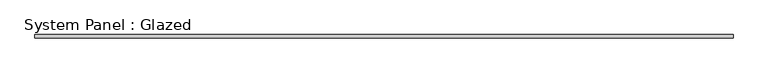
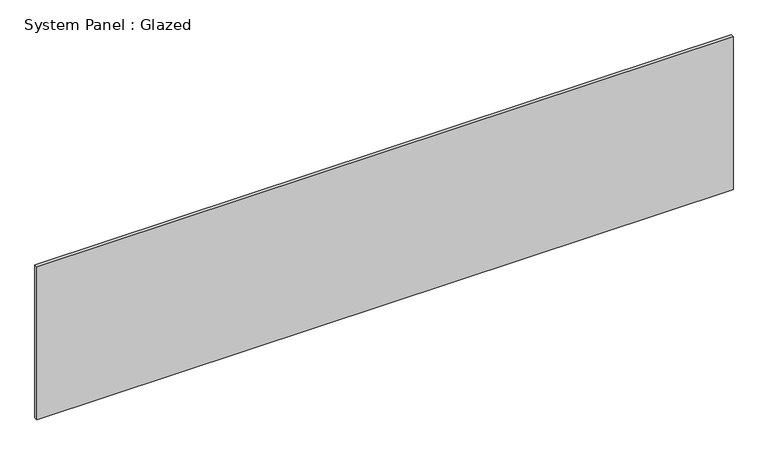
"""IFC4 building model written with IfcOpenShell, lengths in millimetres: plate geometry, System Panel : Glazed."""

from ifc_helpers import new_model, si_unit, origin, origin_with_axes, place, context, project, spatial, polyline, outline, extrude, source, transform, mapped, element, save


def system_panel_glazed_8842d65e(model_context):
    return source(origin(), model_context, "Body", "SweptSolid", [
        extrude(outline(polyline([(2488.4990733, 19.05), (-2488.4990733, 19.05), (-2488.4990733, 44.45), (2488.4990733, 44.45), (2488.4990733, 19.05)])), origin_with_axes(), (0.0, 0.0, 1.0), 1155.7),
    ])


if __name__ == "__main__":
    model = new_model("IFC4")
    model_context = context("Model", 3, world=origin())
    ifc_project = project(units=[si_unit("LENGTHUNIT", "METRE", prefix="MILLI")], contexts=[model_context])
    site = spatial("IfcSite", under=ifc_project)
    building = spatial("IfcBuilding", under=site)
    placement = place(None, origin())
    system_panel_glazed_shape = system_panel_glazed_8842d65e(model_context)
    element("IfcPlate", 1, ObjectType="System Panel : Glazed", at=placement, inside=building, context=model_context, shape_type="MappedRepresentation", body=[
        mapped(system_panel_glazed_shape, transform((0.0, 0.0, 0.0), x_axis=(1.0, 0.0, 0.0), y_axis=(0.0, 1.0, 0.0), z_axis=(0.0, 0.0, 1.0))),
    ])
    save(model, "model.ifc")

# Revit data of these elements
# Type "System Panel : Glazed"
#   Construction Type Id = "GSP4R"
#   Analytic Construction = "1/8 in Pilkington single glazing"
#   Visual Light Transmittance = 0.9
#   Solar Heat Gain Coefficient = 0.86
#   Heat Transfer Coefficient (U) = 1.18115 BTU/(h·ft²·°F)
# Element 1 (IfcPlate, "System Panel : Glazed")
#   Materials on its faces: "Glass"
# Materials
#   "Glass": class "Glass", colour RGB 0 128 192, transparency 0.75, Description = "Soda Lime Glass", Cost = 0
